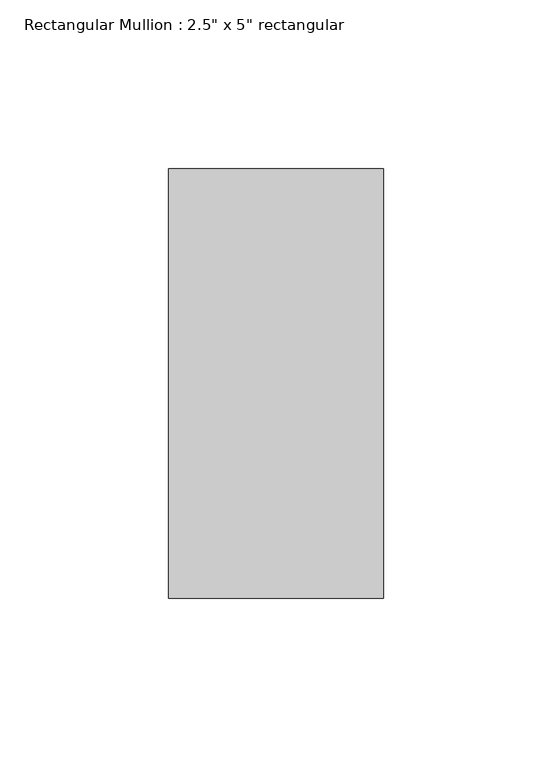
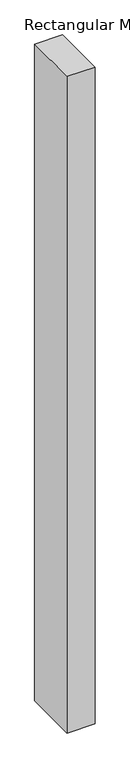
"""IFC4 building model written with IfcOpenShell, lengths in millimetres: member geometry."""

from ifc_helpers import new_model, si_unit, frame, origin, place, context, project, spatial, polyline, outline, extrude, source, transform, mapped, element, save


def member_a8c9f8c2(model_context):
    return source(origin(), model_context, "Body", "SweptSolid", [
        extrude(outline(polyline([(0.0, 63.5), (0.0, -63.5), (-63.5, -63.5), (-63.5, 63.5), (0.0, 63.5)])), frame((0.0, 0.0, -1575.4674874), z_axis=(0.0, 0.0, 1.0), x_axis=(1.0, 0.0, 0.0)), (0.0, 0.0, 1.0), 1575.4674874),
    ])


if __name__ == "__main__":
    model = new_model("IFC4")
    model_context = context("Model", 3, world=origin())
    ifc_project = project(units=[si_unit("LENGTHUNIT", "METRE", prefix="MILLI")], contexts=[model_context])
    site = spatial("IfcSite", under=ifc_project)
    building = spatial("IfcBuilding", under=site)
    placement = place(None, origin())
    member_shape = member_a8c9f8c2(model_context)
    element("IfcMember", 1, ObjectType="Rectangular Mullion : 2.5\" x 5\" rectangular", at=placement, inside=building, context=model_context, shape_type="MappedRepresentation", body=[
        mapped(member_shape, transform((0.0, 0.0, 0.0), x_axis=(1.0, 0.0, 0.0), y_axis=(0.0, 1.0, 0.0), z_axis=(0.0, 0.0, 1.0))),
    ])
    save(model, "model.ifc")

# Revit data of these elements
# Type "Rectangular Mullion : 2.5\" x 5\" rectangular"
#   built-in parameter 1007304 = 0.416667 (stored number, unit not read)
#   built-in parameter 1007301 = 0.104167 (stored number, unit not read)
#   built-in parameter 1007300 = 0.104167 (stored number, unit not read)
# Element 1 (IfcMember, "Rectangular Mullion : 2.5\" x 5\" rectangular")
#   Materials on its faces: "Aluminum"
# Materials
#   "Aluminum": class "Metal", colour RGB 247 247 247, transparency 0, Description = "Aluminum 6061", Cost = 0
